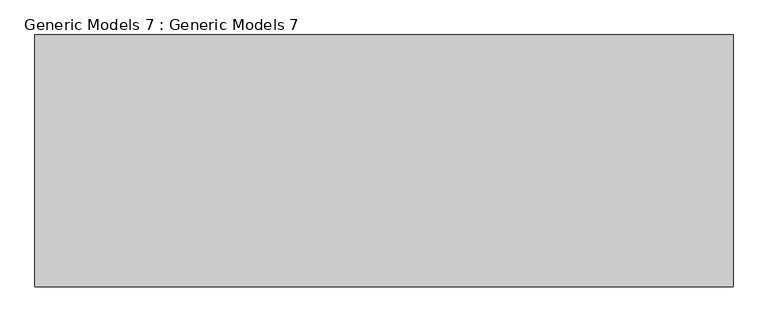
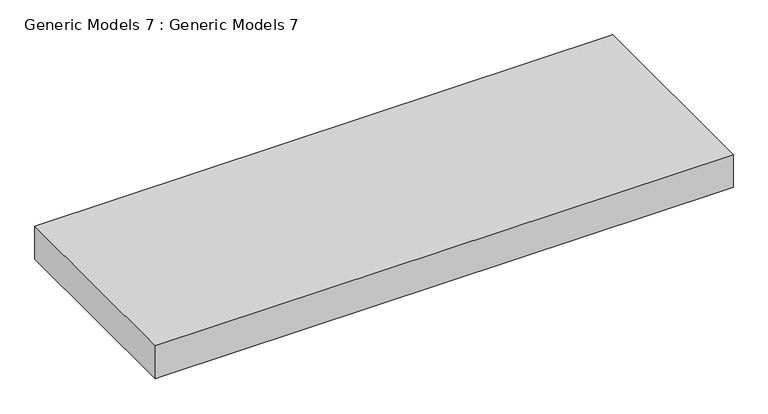
"""IFC4 building model written with IfcOpenShell, lengths in millimetres: proxy geometry, Generic Models 7 : Generic Models 7."""

from ifc_helpers import new_model, si_unit, frame, origin, place, context, project, spatial, polyline, outline, extrude, source, transform, mapped, element, save


def generic_models_7_generic_models_7_8ab6631d(model_context):
    return source(origin(), model_context, "Body", "SweptSolid", [
        extrude(outline(polyline([(2190.75, -3249.7519453), (2190.75, -3224.3519453), (2190.75, -1586.0519453), (2190.75, -1560.6519453), (2292.35, -1560.6519453), (2292.35, -3249.7519453), (2190.75, -3249.7519453)])), frame((0.0, 4276.8444012, 0.0), z_axis=(0.0, 1.0, 0.0), x_axis=(0.0, 0.0, 1.0)), (0.0, 0.0, 1.0), 609.6),
    ])


if __name__ == "__main__":
    model = new_model("IFC4")
    model_context = context("Model", 3, world=origin())
    ifc_project = project(units=[si_unit("LENGTHUNIT", "METRE", prefix="MILLI")], contexts=[model_context])
    site = spatial("IfcSite", under=ifc_project)
    building = spatial("IfcBuilding", under=site)
    placement = place(None, origin())
    generic_models_7_generic_models_7_shape = generic_models_7_generic_models_7_8ab6631d(model_context)
    element("IfcBuildingElementProxy", 1, Name="Generic Models 7 : Generic Models 7", ObjectType="Generic Models 7 : Generic Models 7", at=placement, inside=building, context=model_context, shape_type="MappedRepresentation", body=[
        mapped(generic_models_7_generic_models_7_shape, transform((0.0, 0.0, 0.0), x_axis=(1.0, 0.0, 0.0), y_axis=(0.0, 1.0, 0.0), z_axis=(0.0, 0.0, 1.0))),
    ])
    save(model, "model.ifc")
